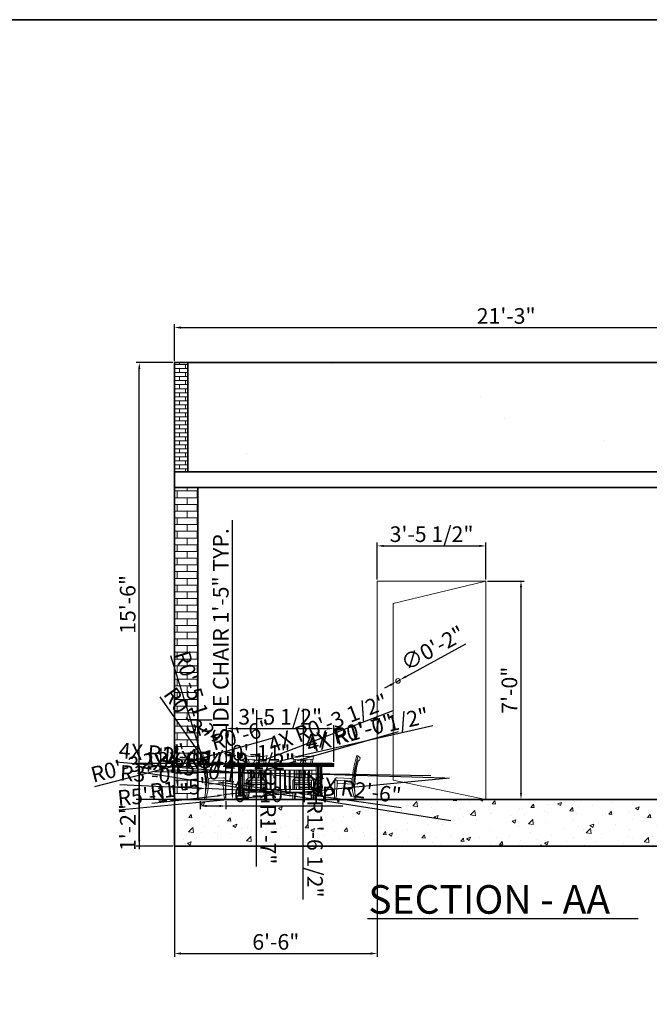
# Model space of a CAD drawing. Units: inches. Extents: x 2656 to 9931, y 1941 to 3068.
# Tile 45 of 46: x 3086 to 3328, y 2689 to 3068. Entities that reach past the tile are written whole.
import ezdxf

# ---------------------------------------------------------------- set-up
doc = ezdxf.new("R2010")
doc.units = ezdxf.units.IN
for name, color, linetype, lineweight in [('A-ANNO-DIMS', 2, 'Continuous', 18), ('A-ANNO-TEXT', 7, 'Continuous', 25), ('A-ANNO-TTLB', 7, 'Continuous', 35), ('A-DOOR', 3, 'Continuous', 18), ('A-FURN', 8, 'Continuous', 13), ('A-SECT', 7, 'Continuous', 35), ('A-SECT-PATT', 251, 'Continuous', 13), ('S-FNDN-PATT', 8, 'Continuous', 13)]:
    doc.layers.add(name, color=color, linetype=linetype, lineweight=lineweight)
doc.styles.get("Standard").update_dxf_attribs({"font": 'arial.ttf'})
doc.dimstyles.new('ISO-25', dxfattribs={"dimtxt": 6, "dimasz": 2.5, "dimexe": 1.25, "dimexo": 0.625, "dimtad": 1, "dimdec": 0, "dimlunit": 3, "dimtxsty": 'Standard', "dimcen": 2.5, "dimadec": 0, "dimazin": 0, "dimtfac": 1, "dimtdec": 0, "dimtmove": 0, "dimatfit": 3, "dimfxl": 1, "dimarcsym": 0})

# ---------------------------------------------------------------- blocks, each defined once
blk = doc.blocks.new('CHAIR-SIDE-ELEV')
for p, q in [((8.87, 8.32), (3.51, 7.95)), ((2.39, 6.89), (1.84, 6.85)), ((1.84, 6.85), (1.84, 5.75)), ((2.37, 5.79), (1.84, 5.75)), ((9.71, 7.4), (3.04, 6.94)), ((8.83, 6.24), (3.07, 5.84)), ((8.83, 7.34), (8.83, 4.83)), ((9.84, -0.04), (9.69, 7.4)), ((9.71, 7.4), (9.84, 7.4)), ((9.84, 6.3), (9.71, 6.3)), ((9.84, 7.4), (9.84, 6.3))]:
    blk.add_line(p, q)
for centre, radius, start, end in [((2.14, 14.23), 2.79, 109.5759, 140.6292), ((3.42, 16.34), 3.46, 185.6828, 203.3447), ((2.56, 9.93), 5.55, 99.4988, 114.6772), ((-4.71, 14.39), 5.87, 8.7526, 22.4843), ((-26.27, 6.8), 28.51, 0.1624, 17.2287), ((-23.21, 7.23), 25.6, 359.491, 18.3244), ((-31.99, 5.96), 34.94, 4.9107, 18.1795), ((-37.8, 4.29), 39.87, 3.6933, 15.7421), ((-15.39, 5.88), 18.46, 341.4048, 9.5718), ((3.67, 7.28), 0.691, 103.5911, 164.2888), ((8.87, 7.48), 0.845, 354.791, 95.2074), ((-23.73, 6.8), 26.12, 344.9035, 0.4566), ((37.9, 2.33), 35.88, 174.4954, 179.8481), ((113.87, 15.79), 105.61, 185.9531, 186.7215), ((26.14, 3.63), 17.15, 180.669, 192.3328)]:
    blk.add_arc(centre, radius, start, end)
blk = doc.blocks.new('*D53')
at = {"layer": 'A-ANNO-DIMS', "color": 0, "lineweight": -2, "transparency": 16777216}
for p, q in [((3167.37, 2784.76), (3167.37, 2875.35)), ((3165.46, 2784.76), (3168.62, 2784.76)), ((3167.37, 2770.36), (3167.37, 2782.26)), ((3165.46, 2767.86), (3168.62, 2767.86))]:
    blk.add_line(p, q, dxfattribs=at)
at = {"layer": 'A-ANNO-DIMS', "color": 0, "transparency": 16777216}
for points in [[(3166.96, 2782.26), (3167.79, 2782.26), (3167.37, 2784.76)], [(3166.96, 2770.36), (3167.79, 2770.36), (3167.37, 2767.86)]]:
    blk.add_solid(points, dxfattribs=at)
at = {"layer": 'Defpoints', "color": 0, "transparency": 16777216}
for p in [(3164.84, 2784.76), (3167.37, 2784.76), (3164.84, 2767.86)]:
    blk.add_point(p, dxfattribs=at)
at = {"layer": 'A-ANNO-DIMS', "color": 0, "transparency": 16777216, "insert": (3163.65, 2831.31), "char_height": 6, "attachment_point": 5, "rotation": 90}
blk.add_mtext('SIDE CHAIR 1\'-5" TYP.', dxfattribs=at)
blk = doc.blocks.new('*D54')
at = {"layer": 'A-ANNO-DIMS', "color": 0, "lineweight": -2, "transparency": 16777216}
for p, q in [((3154.98, 2767.24), (3154.98, 2764.08)), ((3157.48, 2765.33), (3162.34, 2765.33)), ((3164.84, 2767.24), (3164.84, 2764.08)), ((3164.84, 2765.33), (3209.82, 2765.33))]:
    blk.add_line(p, q, dxfattribs=at)
at = {"layer": 'A-ANNO-DIMS', "color": 0, "transparency": 16777216}
for points in [[(3157.48, 2765.75), (3157.48, 2764.91), (3154.98, 2765.33)], [(3162.34, 2765.75), (3162.34, 2764.91), (3164.84, 2765.33)]]:
    blk.add_solid(points, dxfattribs=at)
at = {"layer": 'Defpoints', "color": 0, "transparency": 16777216}
for p in [(3154.98, 2767.86), (3164.84, 2767.86), (3164.84, 2765.33)]:
    blk.add_point(p, dxfattribs=at)
at = {"layer": 'A-ANNO-DIMS', "color": 0, "transparency": 16777216, "insert": (3188.58, 2769.02), "char_height": 6, "attachment_point": 5}
blk.add_mtext('0\'-10" TYP.', dxfattribs=at)
blk = doc.blocks.new('*D89')
at = {"layer": 'A-ANNO-DIMS', "color": 0, "lineweight": -2, "transparency": 16777216}
for p, q in [((3145.05, 2936.52), (3145.05, 2950.64)), ((3147.55, 2949.39), (3397.55, 2949.39)), ((3400.05, 2936.52), (3400.05, 2950.64))]:
    blk.add_line(p, q, dxfattribs=at)
at = {"layer": 'A-ANNO-DIMS', "color": 0, "transparency": 16777216}
for points in [[(3147.55, 2949.81), (3147.55, 2948.98), (3145.05, 2949.39)], [(3397.55, 2949.81), (3397.55, 2948.98), (3400.05, 2949.39)]]:
    blk.add_solid(points, dxfattribs=at)
at = {"layer": 'Defpoints', "color": 0, "transparency": 16777216}
for p in [(3400.05, 2949.39), (3145.05, 2935.89), (3400.05, 2935.89)]:
    blk.add_point(p, dxfattribs=at)
at = {"layer": 'A-ANNO-DIMS', "color": 0, "transparency": 16777216, "insert": (3272.55, 2953.08), "char_height": 6, "attachment_point": 5}
blk.add_mtext('21\'-3"', dxfattribs=at)
blk = doc.blocks.new('*D90')
at = {"layer": 'A-ANNO-DIMS', "color": 0, "lineweight": -2, "transparency": 16777216}
for p, q in [((3144.42, 2935.89), (3130.3, 2935.89)), ((3131.55, 2752.39), (3131.55, 2933.39)), ((3144.42, 2749.89), (3130.3, 2749.89))]:
    blk.add_line(p, q, dxfattribs=at)
at = {"layer": 'A-ANNO-DIMS', "color": 0, "transparency": 16777216}
for points in [[(3131.13, 2933.39), (3131.96, 2933.39), (3131.55, 2935.89)], [(3131.13, 2752.39), (3131.96, 2752.39), (3131.55, 2749.89)]]:
    blk.add_solid(points, dxfattribs=at)
at = {"layer": 'Defpoints', "color": 0, "transparency": 16777216}
for p in [(3131.55, 2935.89), (3145.05, 2935.89), (3145.05, 2749.89)]:
    blk.add_point(p, dxfattribs=at)
at = {"layer": 'A-ANNO-DIMS', "color": 0, "transparency": 16777216, "insert": (3127.86, 2842.89), "char_height": 6, "attachment_point": 5, "rotation": 90}
blk.add_mtext('15\'-6"', dxfattribs=at)
blk = doc.blocks.new('*D95')
at = {"layer": 'A-ANNO-DIMS', "color": 0, "lineweight": -2, "transparency": 16777216}
for p, q in [((3223.02, 2852.52), (3223.02, 2866.64)), ((3225.52, 2865.39), (3262.26, 2865.39)), ((3264.76, 2852.52), (3264.76, 2866.64))]:
    blk.add_line(p, q, dxfattribs=at)
at = {"layer": 'A-ANNO-DIMS', "color": 0, "transparency": 16777216}
for points in [[(3225.52, 2865.81), (3225.52, 2864.98), (3223.02, 2865.39)], [(3262.26, 2865.81), (3262.26, 2864.98), (3264.76, 2865.39)]]:
    blk.add_solid(points, dxfattribs=at)
at = {"layer": 'Defpoints', "color": 0, "transparency": 16777216}
for p in [(3264.76, 2865.39), (3223.02, 2851.89), (3264.76, 2851.89)]:
    blk.add_point(p, dxfattribs=at)
at = {"layer": 'A-ANNO-DIMS', "color": 0, "transparency": 16777216, "insert": (3243.89, 2869.12), "char_height": 6, "attachment_point": 5}
blk.add_mtext('3\'-5 1/2"', dxfattribs=at)
blk = doc.blocks.new('*D96')
at = {"layer": 'A-ANNO-DIMS', "color": 0, "lineweight": -2, "transparency": 16777216}
for p, q in [((3145.05, 2767.27), (3145.05, 2707.33)), ((3223.02, 2767.27), (3223.02, 2707.33)), ((3147.55, 2708.58), (3220.52, 2708.58))]:
    blk.add_line(p, q, dxfattribs=at)
at = {"layer": 'A-ANNO-DIMS', "color": 0, "transparency": 16777216}
for points in [[(3147.55, 2709), (3147.55, 2708.16), (3145.05, 2708.58)], [(3220.52, 2709), (3220.52, 2708.16), (3223.02, 2708.58)]]:
    blk.add_solid(points, dxfattribs=at)
at = {"layer": 'Defpoints', "color": 0, "transparency": 16777216}
for p in [(3145.05, 2767.89), (3223.02, 2767.89), (3223.02, 2708.58)]:
    blk.add_point(p, dxfattribs=at)
at = {"layer": 'A-ANNO-DIMS', "color": 0, "transparency": 16777216, "insert": (3184.03, 2712.27), "char_height": 6, "attachment_point": 5}
blk.add_mtext('6\'-6"', dxfattribs=at)
blk = doc.blocks.new('*D97')
at = {"layer": 'A-ANNO-DIMS', "color": 0, "lineweight": -2, "transparency": 16777216}
for p, q in [((3265.39, 2851.89), (3279.51, 2851.89)), ((3278.26, 2849.39), (3278.26, 2770.39)), ((3265.39, 2767.89), (3279.51, 2767.89))]:
    blk.add_line(p, q, dxfattribs=at)
at = {"layer": 'A-ANNO-DIMS', "color": 0, "transparency": 16777216}
for points in [[(3277.85, 2849.39), (3278.68, 2849.39), (3278.26, 2851.89)], [(3277.85, 2770.39), (3278.68, 2770.39), (3278.26, 2767.89)]]:
    blk.add_solid(points, dxfattribs=at)
at = {"layer": 'Defpoints', "color": 0, "transparency": 16777216}
for p in [(3264.76, 2851.89), (3264.76, 2767.89), (3278.26, 2767.89)]:
    blk.add_point(p, dxfattribs=at)
at = {"layer": 'A-ANNO-DIMS', "color": 0, "transparency": 16777216, "insert": (3274.58, 2809.89), "char_height": 6, "attachment_point": 5, "rotation": 90}
blk.add_mtext('7\'-0"', dxfattribs=at)
blk = doc.blocks.new('*D144')
at = {"layer": 'A-ANNO-DIMS', "color": 0, "lineweight": -2, "transparency": 16777216}
for p, q in [((3165.03, 2782.26), (3165.03, 2796.39)), ((3206.36, 2782.26), (3206.36, 2796.39)), ((3167.53, 2795.14), (3203.86, 2795.14))]:
    blk.add_line(p, q, dxfattribs=at)
at = {"layer": 'A-ANNO-DIMS', "color": 0, "transparency": 16777216}
for points in [[(3167.53, 2795.55), (3167.53, 2794.72), (3165.03, 2795.14)], [(3203.86, 2795.55), (3203.86, 2794.72), (3206.36, 2795.14)]]:
    blk.add_solid(points, dxfattribs=at)
at = {"layer": 'Defpoints', "color": 0, "transparency": 16777216}
for p in [(3206.36, 2795.14), (3165.03, 2781.64), (3206.36, 2781.64)]:
    blk.add_point(p, dxfattribs=at)
at = {"layer": 'A-ANNO-DIMS', "color": 0, "transparency": 16777216, "insert": (3185.7, 2798.87), "char_height": 6, "attachment_point": 5}
blk.add_mtext('3\'-5 1/2"', dxfattribs=at)
blk = doc.blocks.new('*D145')
at = {"layer": 'A-ANNO-DIMS', "color": 0, "lineweight": -2, "transparency": 16777216}
for p, q in [((3205.73, 2781.64), (3130.3, 2781.64)), ((3131.55, 2779.14), (3131.55, 2770.36)), ((3205.93, 2767.86), (3130.3, 2767.86)), ((3131.55, 2767.86), (3131.55, 2748.73))]:
    blk.add_line(p, q, dxfattribs=at)
at = {"layer": 'A-ANNO-DIMS', "color": 0, "transparency": 16777216}
for points in [[(3131.13, 2779.14), (3131.96, 2779.14), (3131.55, 2781.64)], [(3131.13, 2770.36), (3131.96, 2770.36), (3131.55, 2767.86)]]:
    blk.add_solid(points, dxfattribs=at)
at = {"layer": 'Defpoints', "color": 0, "transparency": 16777216}
for p in [(3206.36, 2781.64), (3131.55, 2767.86), (3206.55, 2767.86)]:
    blk.add_point(p, dxfattribs=at)
at = {"layer": 'A-ANNO-DIMS', "color": 0, "transparency": 16777216, "insert": (3127.91, 2757.05), "char_height": 6, "attachment_point": 5, "rotation": 90}
blk.add_mtext('1\'-2"', dxfattribs=at)
blk = doc.blocks.new('*D146')
at = {"layer": 'A-ANNO-DIMS', "color": 0, "lineweight": -2, "transparency": 16777216}
for p, q in [((3154.05, 2768.52), (3154.08, 2782.64)), ((3156.58, 2781.39), (3162.38, 2781.37)), ((3164.84, 2768.49), (3164.88, 2782.61)), ((3164.88, 2781.36), (3189.24, 2781.3))]:
    blk.add_line(p, q, dxfattribs=at)
at = {"layer": 'A-ANNO-DIMS', "color": 0, "transparency": 16777216}
for points in [[(3156.58, 2781.8), (3156.58, 2780.97), (3154.08, 2781.39)], [(3162.38, 2781.79), (3162.37, 2780.95), (3164.88, 2781.36)]]:
    blk.add_solid(points, dxfattribs=at)
at = {"layer": 'Defpoints', "color": 0, "transparency": 16777216}
for p in [(3164.88, 2781.36), (3154.05, 2767.89), (3164.84, 2767.86)]:
    blk.add_point(p, dxfattribs=at)
at = {"layer": 'A-ANNO-DIMS', "color": 0, "transparency": 16777216, "insert": (3178.32, 2785.02), "char_height": 6, "attachment_point": 5, "rotation": 359.846}
blk.add_mtext('0\'-11"', dxfattribs=at)
blk = doc.blocks.new('*D194')
at = {"layer": 'A-ANNO-DIMS', "color": 0, "lineweight": -2, "transparency": 16777216}
for p, q in [((3256.99, 2827.64), (3233.97, 2815.08)), ((3228.02, 2811.82), (3225.82, 2810.63)), ((3230.21, 2813.02), (3231.78, 2813.88))]:
    blk.add_line(p, q, dxfattribs=at)
at = {"layer": 'A-ANNO-DIMS', "color": 0, "transparency": 16777216}
for points in [[(3233.77, 2815.44), (3234.17, 2814.71), (3231.78, 2813.88)], [(3227.82, 2812.19), (3228.22, 2811.46), (3230.21, 2813.02)]]:
    blk.add_solid(points, dxfattribs=at)
at = {"layer": 'Defpoints', "color": 0, "transparency": 16777216}
for p in [(3230.21, 2813.02), (3231.78, 2813.88)]:
    blk.add_point(p, dxfattribs=at)
at = {"layer": 'A-ANNO-DIMS', "color": 0, "transparency": 16777216, "insert": (3244.73, 2825.34), "char_height": 6, "attachment_point": 5, "rotation": 28.6346}
blk.add_mtext('∅0\'-2"', dxfattribs=at)
blk = doc.blocks.new('*D196')
at = {"layer": 'A-ANNO-DIMS', "color": 0, "lineweight": -2, "transparency": 16777216}
for p, q in [((3250.8, 2775.98), (3179.96, 2769.24)), ((3123.72, 2763.89), (3177.47, 2769))]:
    blk.add_line(p, q, dxfattribs=at)
at = {"layer": 'A-ANNO-DIMS', "color": 0, "transparency": 16777216}
blk.add_solid([(3177.43, 2769.42), (3177.51, 2768.59), (3179.96, 2769.24)], dxfattribs=at)
at = {"layer": 'Defpoints', "color": 0, "transparency": 16777216}
for p in [(3250.8, 2775.98), (3179.96, 2769.24)]:
    blk.add_point(p, dxfattribs=at)
at = {"layer": 'A-ANNO-DIMS', "color": 0, "transparency": 16777216, "insert": (3137.11, 2768.87), "char_height": 6, "attachment_point": 5, "rotation": 5.4368}
blk.add_mtext('R5\'-11"', dxfattribs=at)
blk = doc.blocks.new('*D197')
at = {"layer": 'A-ANNO-DIMS', "color": 0, "lineweight": -2, "transparency": 16777216}
for p, q in [((3131.12, 2778.57), (3189.1, 2769.41)), ((3251.24, 2759.6), (3191.57, 2769.02))]:
    blk.add_line(p, q, dxfattribs=at)
at = {"layer": 'A-ANNO-DIMS', "color": 0, "transparency": 16777216}
blk.add_solid([(3189.17, 2769.82), (3189.04, 2769), (3191.57, 2769.02)], dxfattribs=at)
at = {"layer": 'Defpoints', "color": 0, "transparency": 16777216}
for p in [(3191.57, 2769.02), (3251.24, 2759.6)]:
    blk.add_point(p, dxfattribs=at)
at = {"layer": 'A-ANNO-DIMS', "color": 0, "transparency": 16777216, "insert": (3156.35, 2778.36), "char_height": 6, "attachment_point": 5, "rotation": 351.0264}
blk.add_mtext('2X R5\'-0 1/2"', dxfattribs=at)
blk = doc.blocks.new('*D198')
at = {"layer": 'A-ANNO-DIMS', "color": 0, "lineweight": -2, "transparency": 16777216}
for p, q in [((3141.99, 2779.18), (3195.31, 2777.63)), ((3249.14, 2776.06), (3197.81, 2777.55))]:
    blk.add_line(p, q, dxfattribs=at)
at = {"layer": 'A-ANNO-DIMS', "color": 0, "transparency": 16777216}
blk.add_solid([(3195.32, 2778.04), (3195.3, 2777.21), (3197.81, 2777.55)], dxfattribs=at)
at = {"layer": 'Defpoints', "color": 0, "transparency": 16777216}
for p in [(3197.81, 2777.55), (3249.14, 2776.06)]:
    blk.add_point(p, dxfattribs=at)
at = {"layer": 'A-ANNO-DIMS', "color": 0, "transparency": 16777216, "insert": (3167.12, 2782.18), "char_height": 6, "attachment_point": 5, "rotation": 358.3335}
blk.add_mtext('4X R4\'-3 1/2"', dxfattribs=at)
blk = doc.blocks.new('*D199')
at = {"layer": 'A-ANNO-DIMS', "color": 0, "lineweight": -2, "transparency": 16777216}
for p, q in [((3137.54, 2778.61), (3194.5, 2777.68)), ((3243.55, 2776.89), (3197, 2777.64))]:
    blk.add_line(p, q, dxfattribs=at)
at = {"layer": 'A-ANNO-DIMS', "color": 0, "transparency": 16777216}
blk.add_solid([(3194.51, 2778.1), (3194.49, 2777.27), (3197, 2777.64)], dxfattribs=at)
at = {"layer": 'Defpoints', "color": 0, "transparency": 16777216}
for p in [(3197, 2777.64), (3243.55, 2776.89)]:
    blk.add_point(p, dxfattribs=at)
at = {"layer": 'A-ANNO-DIMS', "color": 0, "transparency": 16777216, "insert": (3164.83, 2781.9), "char_height": 6, "attachment_point": 5, "rotation": 359.0709}
blk.add_mtext('3X R3\'-10 1/2"', dxfattribs=at)
blk = doc.blocks.new('*D200')
at = {"layer": 'A-ANNO-DIMS', "color": 0, "lineweight": -2, "transparency": 16777216}
for p, q in [((3124.11, 2773.63), (3154.57, 2772.13)), ((3192.9, 2770.23), (3157.06, 2772))]:
    blk.add_line(p, q, dxfattribs=at)
at = {"layer": 'A-ANNO-DIMS', "color": 0, "transparency": 16777216}
blk.add_solid([(3154.59, 2772.54), (3154.55, 2771.71), (3157.06, 2772)], dxfattribs=at)
at = {"layer": 'Defpoints', "color": 0, "transparency": 16777216}
for p in [(3157.06, 2772), (3192.9, 2770.23)]:
    blk.add_point(p, dxfattribs=at)
at = {"layer": 'A-ANNO-DIMS', "color": 0, "transparency": 16777216, "insert": (3135.74, 2776.75), "char_height": 6, "attachment_point": 5, "rotation": 357.1718}
blk.add_mtext('R3\'-0"', dxfattribs=at)
blk = doc.blocks.new('*D201')
at = {"layer": 'A-ANNO-DIMS', "color": 0, "lineweight": -2, "transparency": 16777216}
for p, q in [((3161.96, 2774.61), (3191.8, 2770.4)), ((3232.26, 2764.68), (3194.27, 2770.05))]:
    blk.add_line(p, q, dxfattribs=at)
at = {"layer": 'A-ANNO-DIMS', "color": 0, "transparency": 16777216}
blk.add_solid([(3194.33, 2770.46), (3194.21, 2769.64), (3191.8, 2770.4)], dxfattribs=at)
at = {"layer": 'Defpoints', "color": 0, "transparency": 16777216}
for p in [(3161.96, 2774.61), (3191.8, 2770.4)]:
    blk.add_point(p, dxfattribs=at)
at = {"layer": 'A-ANNO-DIMS', "color": 0, "transparency": 16777216, "insert": (3215.02, 2770.84), "char_height": 6, "attachment_point": 5, "rotation": 351.9573}
blk.add_mtext('6X R2\'-6"', dxfattribs=at)
blk = doc.blocks.new('*D202')
at = {"layer": 'A-ANNO-DIMS', "color": 0, "lineweight": -2, "transparency": 16777216}
for p, q in [((3176.62, 2802.17), (3176.62, 2783.02)), ((3176.62, 2742.08), (3176.62, 2780.52))]:
    blk.add_line(p, q, dxfattribs=at)
at = {"layer": 'A-ANNO-DIMS', "color": 0, "transparency": 16777216}
blk.add_solid([(3177.03, 2780.52), (3176.2, 2780.52), (3176.62, 2783.02)], dxfattribs=at)
at = {"layer": 'Defpoints', "color": 0, "transparency": 16777216}
for p in [(3176.62, 2802.17), (3176.62, 2783.02)]:
    blk.add_point(p, dxfattribs=at)
at = {"layer": 'A-ANNO-DIMS', "color": 0, "transparency": 16777216, "insert": (3180.26, 2760.05), "char_height": 6, "attachment_point": 5, "rotation": 270.0013}
blk.add_mtext('2X R1\'-7"', dxfattribs=at)
blk = doc.blocks.new('*D203')
at = {"layer": 'A-ANNO-DIMS', "color": 0, "lineweight": -2, "transparency": 16777216}
for p, q in [((3194.58, 2802.71), (3194.58, 2784.3)), ((3194.58, 2729.38), (3194.58, 2781.8))]:
    blk.add_line(p, q, dxfattribs=at)
at = {"layer": 'A-ANNO-DIMS', "color": 0, "transparency": 16777216}
blk.add_solid([(3194.99, 2781.8), (3194.16, 2781.8), (3194.58, 2784.3)], dxfattribs=at)
at = {"layer": 'Defpoints', "color": 0, "transparency": 16777216}
for p in [(3194.58, 2802.71), (3194.58, 2784.3)]:
    blk.add_point(p, dxfattribs=at)
at = {"layer": 'A-ANNO-DIMS', "color": 0, "transparency": 16777216, "insert": (3198.3, 2754.34), "char_height": 6, "attachment_point": 5, "rotation": 270.001}
blk.add_mtext('2X R1\'-6 1/2"', dxfattribs=at)
blk = doc.blocks.new('*D204')
at = {"layer": 'A-ANNO-DIMS', "color": 0, "lineweight": -2, "transparency": 16777216}
for p, q in [((3136.33, 2766.42), (3161.61, 2769.3)), ((3181.14, 2771.53), (3164.09, 2769.59))]:
    blk.add_line(p, q, dxfattribs=at)
at = {"layer": 'A-ANNO-DIMS', "color": 0, "transparency": 16777216}
blk.add_solid([(3161.56, 2769.72), (3161.66, 2768.89), (3164.09, 2769.59)], dxfattribs=at)
at = {"layer": 'Defpoints', "color": 0, "transparency": 16777216}
for p in [(3164.09, 2769.59), (3181.14, 2771.53)]:
    blk.add_point(p, dxfattribs=at)
at = {"layer": 'A-ANNO-DIMS', "color": 0, "transparency": 16777216, "insert": (3147.31, 2771.39), "char_height": 6, "attachment_point": 5, "rotation": 6.4997}
blk.add_mtext('R1\'-5"', dxfattribs=at)
blk = doc.blocks.new('*D205')
at = {"layer": 'A-ANNO-DIMS', "color": 0, "lineweight": -2, "transparency": 16777216}
for p, q in [((3122.56, 2782.38), (3174.92, 2777.86)), ((3194.06, 2776.21), (3177.41, 2777.65))]:
    blk.add_line(p, q, dxfattribs=at)
at = {"layer": 'A-ANNO-DIMS', "color": 0, "transparency": 16777216}
blk.add_solid([(3174.95, 2778.28), (3174.88, 2777.45), (3177.41, 2777.65)], dxfattribs=at)
at = {"layer": 'Defpoints', "color": 0, "transparency": 16777216}
for p in [(3177.41, 2777.65), (3194.06, 2776.21)]:
    blk.add_point(p, dxfattribs=at)
at = {"layer": 'A-ANNO-DIMS', "color": 0, "transparency": 16777216, "insert": (3147.81, 2783.94), "char_height": 6, "attachment_point": 5, "rotation": 355.0718}
blk.add_mtext('4X R1\'-4 1/2"', dxfattribs=at)
blk = doc.blocks.new('*D206')
at = {"layer": 'A-ANNO-DIMS', "color": 0, "lineweight": -2, "transparency": 16777216}
for p, q in [((3231.11, 2793.85), (3194.02, 2783.26)), ((3180.28, 2779.33), (3191.62, 2782.57))]:
    blk.add_line(p, q, dxfattribs=at)
at = {"layer": 'A-ANNO-DIMS', "color": 0, "transparency": 16777216}
blk.add_solid([(3193.91, 2783.66), (3194.14, 2782.86), (3191.62, 2782.57)], dxfattribs=at)
at = {"layer": 'Defpoints', "color": 0, "transparency": 16777216}
for p in [(3191.62, 2782.57), (3180.28, 2779.33)]:
    blk.add_point(p, dxfattribs=at)
at = {"layer": 'A-ANNO-DIMS', "color": 0, "transparency": 16777216, "insert": (3212.76, 2792.44), "char_height": 6, "attachment_point": 5, "rotation": 15.9448}
blk.add_mtext('4X R1\'-0"', dxfattribs=at)
blk = doc.blocks.new('*D207')
at = {"layer": 'A-ANNO-DIMS', "color": 0, "lineweight": -2, "transparency": 16777216}
for p, q in [((3244.41, 2796.17), (3193.18, 2784.45)), ((3183.45, 2782.22), (3190.75, 2783.89))]:
    blk.add_line(p, q, dxfattribs=at)
at = {"layer": 'A-ANNO-DIMS', "color": 0, "transparency": 16777216}
blk.add_solid([(3193.09, 2784.85), (3193.28, 2784.04), (3190.75, 2783.89)], dxfattribs=at)
at = {"layer": 'Defpoints', "color": 0, "transparency": 16777216}
for p in [(3183.45, 2782.22), (3190.75, 2783.89)]:
    blk.add_point(p, dxfattribs=at)
at = {"layer": 'A-ANNO-DIMS', "color": 0, "transparency": 16777216, "insert": (3219.19, 2794.22), "char_height": 6, "attachment_point": 5, "rotation": 12.8892}
blk.add_mtext('4X R0\'-7 1/2"', dxfattribs=at)
blk = doc.blocks.new('*D208')
at = {"layer": 'A-ANNO-DIMS', "color": 0, "lineweight": -2, "transparency": 16777216}
for p, q in [((3182.85, 2791.39), (3158.35, 2784.54)), ((3150.29, 2782.29), (3155.94, 2783.87))]:
    blk.add_line(p, q, dxfattribs=at)
at = {"layer": 'A-ANNO-DIMS', "color": 0, "transparency": 16777216}
blk.add_solid([(3158.24, 2784.94), (3158.46, 2784.14), (3155.94, 2783.87)], dxfattribs=at)
at = {"layer": 'Defpoints', "color": 0, "transparency": 16777216}
for p in [(3150.29, 2782.29), (3155.94, 2783.87)]:
    blk.add_point(p, dxfattribs=at)
at = {"layer": 'A-ANNO-DIMS', "color": 0, "transparency": 16777216, "insert": (3170.81, 2791.86), "char_height": 6, "attachment_point": 5, "rotation": 15.6224}
blk.add_mtext('R0\'-6"', dxfattribs=at)
blk = doc.blocks.new('*D209')
at = {"layer": 'A-ANNO-DIMS', "color": 0, "lineweight": -2, "transparency": 16777216}
for p, q in [((3143.61, 2823.21), (3155.2, 2785.52)), ((3157.56, 2777.83), (3155.93, 2783.13))]:
    blk.add_line(p, q, dxfattribs=at)
at = {"layer": 'A-ANNO-DIMS', "color": 0, "transparency": 16777216}
blk.add_solid([(3155.59, 2785.65), (3154.8, 2785.4), (3155.93, 2783.13)], dxfattribs=at)
at = {"layer": 'Defpoints', "color": 0, "transparency": 16777216}
for p in [(3155.93, 2783.13), (3157.56, 2777.83)]:
    blk.add_point(p, dxfattribs=at)
at = {"layer": 'A-ANNO-DIMS', "color": 0, "transparency": 16777216, "insert": (3152.6, 2806.65), "char_height": 6, "attachment_point": 5, "rotation": 287.0856}
blk.add_mtext('R0\'-5 1/2"', dxfattribs=at)
blk = doc.blocks.new('*D210')
at = {"layer": 'A-ANNO-DIMS', "color": 0, "lineweight": -2, "transparency": 16777216}
for p, q in [((3229.02, 2801.99), (3179.99, 2783.08)), ((3174.27, 2780.87), (3177.65, 2782.18))]:
    blk.add_line(p, q, dxfattribs=at)
at = {"layer": 'A-ANNO-DIMS', "color": 0, "transparency": 16777216}
blk.add_solid([(3179.84, 2783.47), (3180.14, 2782.69), (3177.65, 2782.18)], dxfattribs=at)
at = {"layer": 'Defpoints', "color": 0, "transparency": 16777216}
for p in [(3174.27, 2780.87), (3177.65, 2782.18)]:
    blk.add_point(p, dxfattribs=at)
at = {"layer": 'A-ANNO-DIMS', "color": 0, "transparency": 16777216, "insert": (3204.33, 2796.46), "char_height": 6, "attachment_point": 5, "rotation": 21.087}
blk.add_mtext('4X R0\'-3 1/2"', dxfattribs=at)
blk = doc.blocks.new('*D211')
at = {"layer": 'A-ANNO-DIMS', "color": 0, "lineweight": -2, "transparency": 16777216}
for p, q in [((3158.42, 2784.24), (3155.07, 2783.38)), ((3114.49, 2772.87), (3152.65, 2782.75))]:
    blk.add_line(p, q, dxfattribs=at)
at = {"layer": 'A-ANNO-DIMS', "color": 0, "transparency": 16777216}
blk.add_solid([(3152.55, 2783.15), (3152.75, 2782.35), (3155.07, 2783.38)], dxfattribs=at)
at = {"layer": 'Defpoints', "color": 0, "transparency": 16777216}
for p in [(3158.42, 2784.24), (3155.07, 2783.38)]:
    blk.add_point(p, dxfattribs=at)
at = {"layer": 'A-ANNO-DIMS', "color": 0, "transparency": 16777216, "insert": (3131.42, 2781.11), "char_height": 6, "attachment_point": 5, "rotation": 14.5114}
blk.add_mtext('R0\'-3 1/2"', dxfattribs=at)
blk = doc.blocks.new('*D212')
at = {"layer": 'A-ANNO-DIMS', "color": 0, "lineweight": -2, "transparency": 16777216}
for p, q in [((3139.46, 2807.27), (3154.09, 2786.46)), ((3157.14, 2782.13), (3155.53, 2784.41))]:
    blk.add_line(p, q, dxfattribs=at)
at = {"layer": 'A-ANNO-DIMS', "color": 0, "transparency": 16777216}
blk.add_solid([(3154.43, 2786.7), (3153.75, 2786.22), (3155.53, 2784.41)], dxfattribs=at)
at = {"layer": 'Defpoints', "color": 0, "transparency": 16777216}
for p in [(3155.53, 2784.41), (3157.14, 2782.13)]:
    blk.add_point(p, dxfattribs=at)
at = {"layer": 'A-ANNO-DIMS', "color": 0, "transparency": 16777216, "insert": (3149.08, 2800.01), "char_height": 6, "attachment_point": 5, "rotation": 305.1031}
blk.add_mtext('R0\'-3"', dxfattribs=at)

msp = doc.modelspace()

# ---------------------------------------------------------------- hatches: boundary and pattern name
at = {"layer": 'A-SECT-PATT'}
h = msp.add_hatch(dxfattribs=at)
h.set_pattern_fill('AR-BRSTD', color=256, scale=0.02279243, style=0)
h.paths.add_polyline_path([(3145.05, 2893.89), (3150.15, 2893.89), (3150.15, 2935.89), (3145.05, 2935.89)])
h = msp.add_hatch(dxfattribs=at)
h.set_pattern_fill('AR-SAND', color=256, scale=2)
h.set_pattern_definition([(37.5, (0, 64.96), (-3.2, 97.8826), [0, -77.216, 0, -86.36, 0, -82.55]), (7.5, (0, 64.96), (89.9047, 143.365), [0, -41.656, 0, -69.596, 0, -26.67]), (327.5, (-62.48, 64.96), (158.1985, 0.2874), [0, -25.4, 0, -91.44, 0, -119.38]), (317.5, (-62.48, 64.96), (152.7113, 44.586), [0, -12.7, 0, -59.944, 0, -68.58])])
h.paths.add_polyline_path([(3394.03, 2893.89), (3394.03, 2935.89), (3150.15, 2935.89), (3150.15, 2893.89)])
h = msp.add_hatch(dxfattribs=at)
h.set_pattern_fill('AR-BRSTD', color=256, scale=0.03818174, style=0)
h.paths.add_polyline_path([(3145.05, 2767.89), (3154.05, 2767.89), (3154.05, 2887.89), (3145.05, 2887.89)])
at = {"layer": 'S-FNDN-PATT'}
h = msp.add_hatch(dxfattribs=at)
h.set_pattern_fill('AR-CONC', color=256, scale=0.082, style=0)
h.paths.add_polyline_path([(3145.05, 2749.89), (3400.05, 2749.89), (3400.05, 2767.89), (3145.05, 2767.89)])

# ---------------------------------------------------------------- linework, layer by layer
at = {"layer": 'A-ANNO-TEXT'}
msp.add_line((3219.25, 2722.08), (3323.27, 2722.08), dxfattribs=at)
at = {"layer": 'A-ANNO-TTLB'}
msp.add_lwpolyline([(2655.77, 3067.84), (3515.43, 3067.84), (3515.43, 1940.89), (2655.77, 1940.89)], close=True, dxfattribs=at)
at = {"layer": 'A-DOOR'}
for p, q in [((3223.02, 2851.89), (3264.76, 2851.89)), ((3223.02, 2851.89), (3223.02, 2767.89)), ((3264.76, 2851.89), (3229.09, 2843.24)), ((3264.76, 2851.89), (3264.76, 2767.89)), ((3264.76, 2851.89), (3264.76, 2851.89)), ((3229.09, 2843.24), (3229.09, 2775.24)), ((3229.09, 2775.24), (3264.76, 2767.89))]:
    msp.add_line(p, q, dxfattribs=at)
msp.add_lwpolyline([(3223.02, 2851.89), (3264.76, 2851.89), (3264.76, 2767.89), (3223.02, 2767.89)], close=True, dxfattribs=at)
msp.add_circle((3230.99, 2813.45), 0.891, dxfattribs=at)
at = {"layer": 'A-FURN'}
for p, q in [((3206.36, 2781.64), (3165.03, 2781.64)), ((3206.36, 2780.54), (3165.03, 2780.54)), ((3169.63, 2780.54), (3169.63, 2769.51)), ((3170.02, 2769.51), (3170.02, 2780.54)), ((3170.47, 2769.51), (3170.47, 2780.54)), ((3170.92, 2769.51), (3170.92, 2780.54)), ((3171.38, 2769.51), (3171.38, 2780.54)), ((3171.83, 2780.54), (3171.83, 2769.51)), ((3199.56, 2780.54), (3199.56, 2769.51)), ((3200.01, 2769.51), (3200.01, 2780.54)), ((3200.47, 2769.51), (3200.47, 2780.54)), ((3200.92, 2769.51), (3200.92, 2780.54)), ((3201.37, 2769.51), (3201.37, 2780.54)), ((3201.76, 2780.54), (3201.76, 2769.51)), ((3199.56, 2779.07), (3171.83, 2779.07)), ((3174.49, 2771.72), (3174.49, 2779.07)), ((3174.86, 2771.72), (3174.86, 2779.07)), ((3176.33, 2771.72), (3176.33, 2779.07)), ((3176.7, 2771.72), (3176.7, 2779.07)), ((3178.17, 2771.72), (3178.17, 2779.07)), ((3178.53, 2771.72), (3178.53, 2779.07)), ((3180, 2771.72), (3180, 2779.07)), ((3180.37, 2771.72), (3180.37, 2779.07)), ((3181.84, 2771.72), (3181.84, 2779.07)), ((3182.21, 2771.72), (3182.21, 2779.07)), ((3183.68, 2771.72), (3183.68, 2779.07)), ((3184.04, 2771.72), (3184.04, 2779.07)), ((3185.51, 2771.72), (3185.51, 2779.07)), ((3185.88, 2771.72), (3185.88, 2779.07)), ((3187.35, 2771.72), (3187.35, 2779.07)), ((3187.72, 2771.72), (3187.72, 2779.07)), ((3189.18, 2771.72), (3189.18, 2779.07)), ((3189.55, 2771.72), (3189.55, 2779.07)), ((3191.02, 2771.72), (3191.02, 2779.07)), ((3191.39, 2771.72), (3191.39, 2779.07)), ((3192.86, 2771.72), (3192.86, 2779.07)), ((3193.23, 2771.72), (3193.23, 2779.07)), ((3194.69, 2771.72), (3194.69, 2779.07)), ((3195.06, 2771.72), (3195.06, 2779.07)), ((3196.53, 2771.72), (3196.53, 2779.07)), ((3196.9, 2771.72), (3196.9, 2779.07)), ((3174.49, 2775.3), (3172.67, 2775.3)), ((3174.49, 2774.2), (3173.4, 2774.2)), ((3174.49, 2773.65), (3173.42, 2773.65)), ((3174.49, 2776.22), (3173.93, 2776.22)), ((3176.33, 2776.22), (3174.86, 2776.22)), ((3176.33, 2775.3), (3174.86, 2775.3)), ((3176.33, 2774.2), (3174.86, 2774.2)), ((3176.33, 2773.65), (3174.86, 2773.65)), ((3178.17, 2776.22), (3176.7, 2776.22)), ((3178.17, 2775.3), (3176.7, 2775.3)), ((3178.17, 2774.2), (3176.7, 2774.2)), ((3178.17, 2773.65), (3176.7, 2773.65)), ((3179.31, 2776.22), (3178.53, 2776.22)), ((3180, 2775.3), (3178.53, 2775.3)), ((3179.83, 2774.2), (3178.53, 2774.2)), ((3179.83, 2773.65), (3178.53, 2773.65)), ((3180.57, 2775.3), (3180.37, 2775.3)), ((3191.02, 2775.3), (3190.63, 2775.3)), ((3192.86, 2774.2), (3191.36, 2774.2)), ((3192.86, 2773.65), (3191.38, 2773.65)), ((3192.86, 2775.3), (3191.39, 2775.3)), ((3192.86, 2776.22), (3191.89, 2776.22)), ((3194.69, 2776.22), (3193.23, 2776.22)), ((3194.69, 2775.3), (3193.23, 2775.3)), ((3194.69, 2774.2), (3193.23, 2774.2)), ((3194.69, 2773.65), (3193.23, 2773.65)), ((3196.53, 2776.22), (3195.06, 2776.22)), ((3196.53, 2775.3), (3195.06, 2775.3)), ((3196.53, 2774.2), (3195.06, 2774.2)), ((3196.53, 2773.65), (3195.06, 2773.65)), ((3197.26, 2776.22), (3196.9, 2776.22)), ((3198.52, 2775.3), (3196.9, 2775.3)), ((3197.79, 2774.2), (3196.9, 2774.2)), ((3197.79, 2773.65), (3196.9, 2773.65)), ((3169.17, 2769.12), (3172.38, 2769.12)), ((3169.53, 2769.51), (3171.92, 2769.51)), ((3169.53, 2769.4), (3169.53, 2769.51)), ((3169.53, 2769.4), (3171.92, 2769.4)), ((3199.56, 2771.72), (3171.83, 2771.72)), ((3199.56, 2770.62), (3171.83, 2770.62)), ((3171.92, 2769.4), (3171.92, 2769.51)), ((3172.29, 2769.12), (3172.29, 2769.18)), ((3199.1, 2769.12), (3199.1, 2769.18)), ((3199.47, 2769.51), (3201.86, 2769.51)), ((3199.47, 2769.4), (3199.47, 2769.51)), ((3199.47, 2769.4), (3201.86, 2769.4)), ((3201.86, 2769.4), (3201.86, 2769.51)), ((3202.22, 2769.12), (3202.22, 2769.18))]:
    msp.add_line(p, q, dxfattribs=at)
for points in [[(3173.08, 2781.87, 0.005505), (3172.94, 2782.99, 0.060823), (3172.53, 2784.76)], [(3180.16, 2781.84, -0.00565), (3180.3, 2782.99, -0.060823), (3180.7, 2784.76)], [(3191.04, 2781.84, 0.005652), (3190.89, 2782.99, 0.060823), (3190.49, 2784.76)], [(3198.12, 2781.87, -0.00551), (3198.26, 2782.99, -0.060823), (3198.66, 2784.76)], [(3173.84, 2781.87, 0.031241), (3173.43, 2783.28)], [(3177.76, 2781.85, 0.048013), (3177.51, 2782.5, 0.26274), (3176.62, 2783.01, 0.26274), (3175.72, 2782.5, 0.047326), (3175.47, 2781.86)], [(3179.39, 2781.84, -0.031747), (3179.8, 2783.28)], [(3191.8, 2781.84, 0.031759), (3191.39, 2783.28)], [(3195.72, 2781.86, 0.047392), (3195.47, 2782.5, 0.26274), (3194.58, 2783.01, 0.26274), (3193.68, 2782.5, 0.048065), (3193.43, 2781.85)], [(3197.35, 2781.87, -0.031264), (3197.76, 2783.28)], [(3173.41, 2776.04, 0.01476), (3173.32, 2779.07)], [(3174.19, 2776.22, 0.015292), (3174.15, 2779.07)], [(3175.64, 2779.07, -0.042829), (3175.89, 2776.22)], [(3177.35, 2776.22, -0.042829), (3177.59, 2779.07)], [(3179.04, 2776.22, -0.015292), (3179.09, 2779.07)], [(3179.83, 2776.04, -0.01476), (3179.92, 2779.07)], [(3192.15, 2776.22, 0.015292), (3192.11, 2779.07)], [(3193.6, 2779.07, -0.042829), (3193.85, 2776.22)], [(3195.3, 2776.22, -0.042829), (3195.55, 2779.07)], [(3197, 2776.22, -0.015292), (3197.04, 2779.07)], [(3197.79, 2776.04, -0.01476), (3197.88, 2779.07)], [(3174.13, 2774.2, -0.020607), (3173.99, 2771.72)], [(3179.1, 2774.2, 0.020607), (3179.24, 2771.72)], [(3192.09, 2774.2, -0.020607), (3191.95, 2771.72)], [(3197.06, 2774.2, 0.020607), (3197.2, 2771.72)], [(3173.87, 2770.62, -0.003701), (3173.81, 2770.18, 0.009693), (3173.44, 2767.86), (3172.67, 2767.86), (3172.67, 2770.62)], [(3173.13, 2767.86, 0.009723), (3173.39, 2770.62)], [(3179.37, 2770.62, 0.003701), (3179.43, 2770.18, -0.009693), (3179.79, 2767.86), (3180.57, 2767.86), (3180.57, 2770.62)], [(3180.11, 2767.86, -0.009723), (3179.84, 2770.62)], [(3191.83, 2770.62, -0.003701), (3191.76, 2770.18, 0.009693), (3191.4, 2767.86), (3190.63, 2767.86), (3190.63, 2770.62)], [(3191.09, 2767.86, 0.009723), (3191.35, 2770.62)], [(3197.33, 2770.62, 0.003701), (3197.39, 2770.18, -0.009693), (3197.75, 2767.86), (3198.52, 2767.86), (3198.52, 2770.62)], [(3198.07, 2767.86, -0.009723), (3197.8, 2770.62)]]:
    msp.add_lwpolyline(points, format="xyb", dxfattribs=at)
for points in [[(3165.03, 2781.64), (3165.03, 2781.31), (3206.36, 2781.31)], [(3206.36, 2780.87), (3165.03, 2780.87), (3165.03, 2780.54)], [(3165.4, 2781.31), (3165.4, 2780.87)], [(3205.99, 2781.31), (3205.99, 2780.87)], [(3206.36, 2781.64), (3206.36, 2781.31)], [(3206.36, 2780.87), (3206.36, 2780.54)], [(3172.67, 2771.72), (3172.67, 2775.3)], [(3173.4, 2771.72), (3173.4, 2775.3)], [(3179.83, 2771.72), (3179.83, 2775.3)], [(3180.57, 2771.72), (3180.57, 2775.3)], [(3190.63, 2771.72), (3190.63, 2775.3)], [(3197.79, 2771.72), (3197.79, 2775.3)], [(3198.52, 2771.72), (3198.52, 2775.3)], [(3172.38, 2769.12), (3172.38, 2767.86), (3169.17, 2767.86), (3169.17, 2769.18)], [(3202.32, 2769.12), (3199.01, 2769.12), (3199.01, 2767.86)], [(3202.32, 2769.12), (3202.32, 2767.86), (3199.01, 2767.86)]]:
    msp.add_lwpolyline(points, dxfattribs=at)
for points in [[(3175.67, 2783.04), (3175.96, 2783.04), (3175.96, 2782.77), (3175.67, 2782.77)], [(3175.72, 2782.98), (3175.9, 2782.98), (3175.9, 2782.83), (3175.72, 2782.83)], [(3177.57, 2783.04), (3177.28, 2783.04), (3177.28, 2782.77), (3177.57, 2782.77)], [(3177.51, 2782.98), (3177.33, 2782.98), (3177.33, 2782.83), (3177.51, 2782.83)], [(3193.63, 2783.04), (3193.92, 2783.04), (3193.92, 2782.77), (3193.63, 2782.77)], [(3193.68, 2782.98), (3193.86, 2782.98), (3193.86, 2782.83), (3193.68, 2782.83)], [(3195.52, 2783.04), (3195.23, 2783.04), (3195.23, 2782.77), (3195.52, 2782.77)], [(3195.47, 2782.98), (3195.29, 2782.98), (3195.29, 2782.83), (3195.47, 2782.83)]]:
    msp.add_lwpolyline(points, close=True, dxfattribs=at)
for centre, radius, start, end in [((3176.62, 2802.71), 18.41, 257.1783, 282.8217), ((3194.58, 2802.71), 18.41, 257.1783, 282.8217), ((3176.62, 2802.17), 19.15, 258.7604, 281.2396), ((3194.58, 2802.17), 19.15, 258.7604, 281.2396), ((3174.13, 2774.82), 1.41, 98.0081, 160.1385), ((3179.11, 2774.82), 1.41, 50.7994, 81.9919), ((3179.11, 2774.82), 1.41, 19.8615, 26.8443), ((3192.08, 2774.82), 1.41, 138.7966, 160.1385), ((3192.08, 2774.82), 1.41, 98.0081, 119.4837), ((3197.07, 2774.82), 1.41, 19.8615, 81.9919), ((3169.63, 2769), 0.41, 103.1674, 154.1522), ((3171.83, 2769), 0.41, 25.8478, 76.8326), ((3199.56, 2769), 0.41, 103.1674, 154.1522), ((3201.76, 2769), 0.41, 25.8478, 76.8326)]:
    msp.add_arc(centre, radius, start, end, dxfattribs=at)
at = {"layer": 'A-SECT'}
for p, q in [((3145.05, 2935.89), (3145.05, 2749.89)), ((3145.05, 2935.89), (3400.05, 2935.89)), ((3150.15, 2893.89), (3150.15, 2935.89)), ((3145.05, 2893.89), (3400.05, 2893.89)), ((3145.05, 2887.89), (3400.05, 2887.89)), ((3154.05, 2887.89), (3154.05, 2767.89)), ((3145.05, 2767.89), (3400.05, 2767.89)), ((3145.05, 2749.89), (3400.05, 2749.89)), ((3145.05, 2749.89), (3400.05, 2749.89))]:
    msp.add_line(p, q, dxfattribs=at)

# ---------------------------------------------------------------- block references
at = {"layer": 'A-FURN'}
msp.add_blockref('CHAIR-SIDE-ELEV', (3155, 2767.9), dxfattribs=at)
at = {"layer": 'A-FURN', "extrusion": (0, 0, -1), "zscale": -1}
msp.add_blockref('CHAIR-SIDE-ELEV', (-3216.39, 2767.9), dxfattribs=at)

# ---------------------------------------------------------------- texts
at = {"layer": 'A-ANNO-TEXT', "insert": (3219.59, 2734.88), "char_height": 11, "attachment_point": 1}
msp.add_mtext_dynamic_manual_height_columns('SECTION - AA', width=240.1741, gutter_width=12.5, heights=[0], dxfattribs=at)

# ---------------------------------------------------------------- dimensions: what is measured, and where the dimension line sits
at = {"layer": 'A-ANNO-DIMS'}
for base, p1, p2, picture, middle in [((3400.05, 2949.39), (3145.05, 2935.89), (3400.05, 2935.89), '*D89', (3272.55, 2953.08)), ((3264.76, 2865.39), (3223.02, 2851.89), (3264.76, 2851.89), '*D95', (3243.89, 2869.12)), ((3206.36, 2795.14), (3165.03, 2781.64), (3206.36, 2781.64), '*D144', (3185.7, 2798.87)), ((3223.02, 2708.58), (3145.05, 2767.89), (3223.02, 2767.89), '*D96', (3184.03, 2712.27))]:
    dim = msp.add_linear_dim(base=base, p1=p1, p2=p2, dimstyle='ISO-25', override={"dimdec": 1, "dimlfac": 1, "dimrnd": 0, "dimzin": 1, "dimdsep": 46, "dimlunit": 4, "dimfrac": 2}, dxfattribs=at)
    dim.commit()
    dim.dimension.update_dxf_attribs({"geometry": picture, "text_midpoint": middle})
for base, p1, p2, angle, picture, middle in [((3131.55, 2935.89), (3145.05, 2749.89), (3145.05, 2935.89), 90, '*D90', (3127.86, 2842.89)), ((3278.26, 2767.89), (3264.76, 2851.89), (3264.76, 2767.89), 270, '*D97', (3274.58, 2809.89)), ((3164.88, 2781.36), (3154.05, 2767.89), (3164.84, 2767.86), 359.846, '*D146', (3178.32, 2785.02)), ((3131.55, 2767.86), (3206.36, 2781.64), (3206.55, 2767.86), 90, '*D145', (3127.91, 2757.05))]:
    dim = msp.add_linear_dim(base=base, p1=p1, p2=p2, angle=angle, dimstyle='ISO-25', override={"dimdec": 1, "dimlfac": 1, "dimrnd": 0, "dimzin": 1, "dimdsep": 46, "dimlunit": 4, "dimfrac": 2}, dxfattribs=at)
    dim.commit()
    dim.dimension.update_dxf_attribs({"geometry": picture, "text_midpoint": middle})
dim = msp.add_linear_dim(base=(3167.37, 2784.76), p1=(3164.84, 2767.86), p2=(3164.84, 2784.76), angle=90, text='SIDE CHAIR <> TYP.', dimstyle='ISO-25', override={"dimdec": 1, "dimlfac": 1, "dimrnd": 0, "dimzin": 1, "dimdsep": 46, "dimlunit": 4, "dimfrac": 2}, dxfattribs=at)
dim.commit()
dim.dimension.update_dxf_attribs({"geometry": '*D53', "text_midpoint": (3163.65, 2831.31)})
dim = msp.add_diameter_dim_2p(p1=(3230.21, 2813.02), p2=(3231.78, 2813.88), dimstyle='ISO-25', override={"dimdec": 1, "dimlfac": 1, "dimrnd": 0, "dimzin": 1, "dimdsep": 46, "dimlunit": 4, "dimfrac": 2}, dxfattribs=at)
dim.commit()
dim.dimension.update_dxf_attribs({"geometry": '*D194', "text_midpoint": (3246.58, 2821.96)})
for center, mpoint, picture, middle in [((3157.56, 2777.83), (3155.93, 2783.13), '*D209', (3152.6, 2806.65)), ((3157.14, 2782.13), (3155.53, 2784.41), '*D212', (3149.08, 2800.01)), ((3150.29, 2782.29), (3155.94, 2783.87), '*D208', (3170.81, 2791.86)), ((3158.42, 2784.24), (3155.07, 2783.38), '*D211', (3131.42, 2781.11)), ((3181.14, 2771.53), (3164.09, 2769.59), '*D204', (3147.31, 2771.39))]:
    dim = msp.add_radius_dim(center=center, mpoint=mpoint, dimstyle='ISO-25', override={"dimdec": 1, "dimlfac": 1, "dimrnd": 0, "dimzin": 1, "dimdsep": 46, "dimlunit": 4, "dimfrac": 2}, dxfattribs=at)
    dim.commit()
    dim.dimension.update_dxf_attribs({"geometry": picture, "text_midpoint": middle})
for center, mpoint, text, picture, middle in [((3174.27, 2780.87), (3177.65, 2782.18), '4X <>', '*D210', (3204.33, 2796.46)), ((3183.45, 2782.22), (3190.75, 2783.89), '4X <>', '*D207', (3219.19, 2794.22)), ((3180.28, 2779.33), (3191.62, 2782.57), '4X <>', '*D206', (3212.76, 2792.44)), ((3176.6176, 2802.1666), (3176.618, 2783.0155), '2X <>', '*D202', (3180.2579, 2760.0474)), ((3194.58, 2802.71), (3194.58, 2784.3), '2X <>', '*D203', (3198.3, 2754.34)), ((3194.06, 2776.21), (3177.41, 2777.65), '4X <>', '*D205', (3147.81, 2783.94)), ((3243.55, 2776.89), (3197, 2777.64), '3X <>', '*D199', (3164.83, 2781.9)), ((3161.96, 2774.61), (3191.8, 2770.4), '6X <>', '*D201', (3215.02, 2770.84))]:
    dim = msp.add_radius_dim(center=center, mpoint=mpoint, text=text, dimstyle='ISO-25', override={"dimdec": 1, "dimlfac": 1, "dimrnd": 0, "dimzin": 1, "dimdsep": 46, "dimlunit": 4, "dimfrac": 2}, dxfattribs=at)
    dim.commit()
    dim.dimension.update_dxf_attribs({"geometry": picture, "text_midpoint": middle})
for center, mpoint, text, picture, middle in [((3249.14, 2776.06), (3197.81, 2777.55), '4X <>', '*D198', (3167.01, 2778.45)), ((3251.24, 2759.6), (3191.57, 2769.02), '2X <>', '*D197', (3155.77, 2774.68))]:
    dim = msp.add_radius_dim(center=center, mpoint=mpoint, text=text, dimstyle='ISO-25', override={"dimdec": 1, "dimlfac": 1, "dimrnd": 0, "dimzin": 1, "dimdsep": 46, "dimlunit": 4, "dimfrac": 2}, dxfattribs=at)
    dim.commit()
    dim.dimension.update_dxf_attribs({"geometry": picture, "text_midpoint": middle, "dimtype": 164})
for center, mpoint, picture, middle in [((3192.9, 2770.23), (3157.06, 2772), '*D200', (3135.56, 2773.06)), ((3250.8, 2775.98), (3179.96, 2769.24), '*D196', (3137.46, 2765.19))]:
    dim = msp.add_radius_dim(center=center, mpoint=mpoint, dimstyle='ISO-25', override={"dimdec": 1, "dimlfac": 1, "dimrnd": 0, "dimzin": 1, "dimdsep": 46, "dimlunit": 4, "dimfrac": 2}, dxfattribs=at)
    dim.commit()
    dim.dimension.update_dxf_attribs({"geometry": picture, "text_midpoint": middle, "dimtype": 164})
dim = msp.add_linear_dim(base=(3164.84, 2765.33), p1=(3154.98, 2767.86), p2=(3164.84, 2767.86), text='<> TYP.', dimstyle='ISO-25', override={"dimdec": 1, "dimlfac": 1, "dimrnd": 0, "dimzin": 1, "dimdsep": 46, "dimlunit": 4, "dimfrac": 2}, dxfattribs=at)
dim.commit()
dim.dimension.update_dxf_attribs({"geometry": '*D54', "text_midpoint": (3188.58, 2769.02)})

doc.saveas('drawing.dxf')
